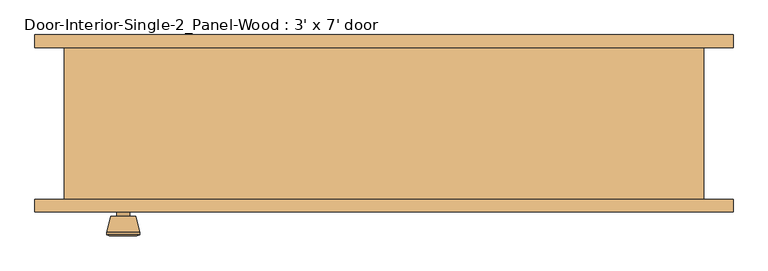
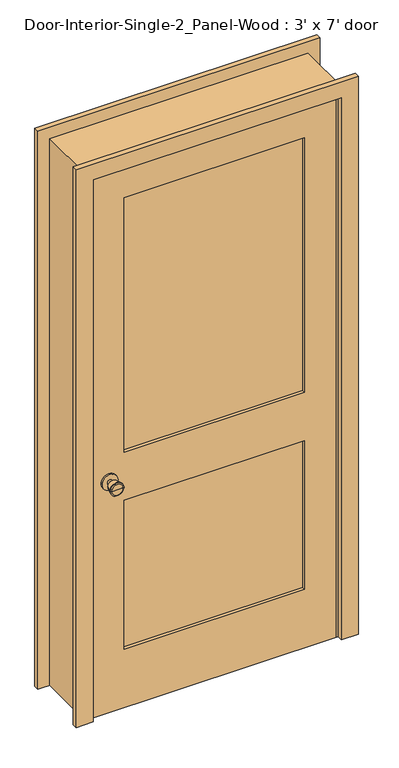
"""IFC4 building model written with IfcOpenShell, lengths in millimetres: door geometry, Door-Interior-Single-2_Panel-Wood : 3' x 7' door."""

from ifc_helpers import new_model, si_unit, point, frame, frame_2d, origin, place, context, project, spatial, polyline, circle_curve, trimmed, segment, composite_curve, outline, extrude, faceted_brep, source, transform, mapped, element, save
from ifc_brep_helpers import plane_surface, cylinder_surface, revolved_surface, advanced_brep


def door_interior_single_2_panel_wood_3_x_7_door_700963f9(model_context):
    return source(origin(), model_context, "Body", "SolidModel", [
        advanced_brep(
        [(-393.7, -70.9, 914.4), (-403.7, -70.9, 914.4), (-383.7, -70.9, 914.4), (-373.2241324, -21.9, 914.4), (-414.1758676, -21.9, 914.4), (-393.7, -21.9, 914.4), (-368.7, -23.7278681, 914.4), (-418.7, -23.7278681, 914.4), (-368.7, -27.1915463, 914.4), (-418.7, -27.1915463, 914.4), (-375.063764, -51.9, 914.4), (-412.336236, -51.9, 914.4), (-383.7, -51.9, 914.4), (-403.7, -51.9, 914.4)],
        [
            (0, 1),
            (1, 2, circle_curve(frame((-393.7, -70.9, 914.4), z_axis=(0.0, -1.0, 0.0), x_axis=(-1.0, 0.0, 0.0)), 10.0)),
            (2, 0),
            (2, 1, circle_curve(frame((-393.7, -70.9, 914.4), z_axis=(0.0, -1.0, 0.0), x_axis=(-1.0, 0.0, 0.0)), 10.0)),
            (3, 4, circle_curve(frame((-393.7, -21.9, 914.4), z_axis=(0.0, 1.0, 0.0), x_axis=(-1.0, 0.0, 0.0)), 20.4758676)),
            (4, 5),
            (5, 3),
            (4, 3, circle_curve(frame((-393.7, -21.9, 914.4), z_axis=(0.0, 1.0, 0.0), x_axis=(-1.0, 0.0, 0.0)), 20.4758676)),
            (6, 7, circle_curve(frame((-393.7, -23.7278681, 914.4), z_axis=(0.0, 1.0, 0.0), x_axis=(-1.0, 0.0, 0.0)), 25.0)),
            (7, 4),
            (3, 6),
            (7, 6, circle_curve(frame((-393.7, -23.7278681, 914.4), z_axis=(0.0, 1.0, 0.0), x_axis=(-1.0, 0.0, 0.0)), 25.0)),
            (8, 9, circle_curve(frame((-393.7, -27.1915463, 914.4), z_axis=(0.0, 1.0, 0.0), x_axis=(-1.0, 0.0, 0.0)), 25.0)),
            (9, 7),
            (6, 8),
            (9, 8, circle_curve(frame((-393.7, -27.1915463, 914.4), z_axis=(0.0, 1.0, 0.0), x_axis=(-1.0, 0.0, 0.0)), 25.0)),
            (10, 11, circle_curve(frame((-393.7, -51.9, 914.4), z_axis=(0.0, 1.0, 0.0), x_axis=(-1.0, 0.0, 0.0)), 18.636236)),
            (11, 9),
            (8, 10),
            (11, 10, circle_curve(frame((-393.7, -51.9, 914.4), z_axis=(0.0, 1.0, 0.0), x_axis=(-1.0, 0.0, 0.0)), 18.636236)),
            (12, 13, circle_curve(frame((-393.7, -51.9, 914.4), z_axis=(0.0, 1.0, 0.0), x_axis=(-1.0, 0.0, 0.0)), 10.0)),
            (13, 11),
            (10, 12),
            (13, 12, circle_curve(frame((-393.7, -51.9, 914.4), z_axis=(0.0, 1.0, 0.0), x_axis=(-1.0, 0.0, 0.0)), 10.0)),
            (1, 13),
            (12, 2),
        ],
        [
            plane_surface(frame((-393.7, -70.9, 914.4), z_axis=(0.0, -1.0, 0.0), x_axis=(-1.0, 0.0, 0.0))),
            plane_surface(frame((-393.7, -21.9, 914.4), z_axis=(0.0, 1.0, 0.0), x_axis=(-1.0, 0.0, 0.0))),
            revolved_surface(polyline([(-414.1758676, -21.9, 914.4), (-418.7, -23.7278681, 914.4)]), (-393.7, -70.9, 914.4), (0.0, -1.0, 0.0)),
            cylinder_surface(frame((-393.7, -70.9, 914.4), z_axis=(0.0, -1.0, 0.0), x_axis=(-1.0, 0.0, 0.0)), 25.0),
            revolved_surface(polyline([(-418.7, -27.1915463, 914.4), (-412.336236, -51.9, 914.4)]), (-393.7, -70.9, 914.4), (0.0, -1.0, 0.0)),
            plane_surface(frame((-393.7, -51.9, 914.4), z_axis=(0.0, -1.0, 0.0), x_axis=(-1.0, 0.0, 0.0))),
            cylinder_surface(frame((-393.7, -70.9, 914.4), z_axis=(0.0, -1.0, 0.0), x_axis=(-1.0, 0.0, 0.0)), 10.0),
        ],
        [
            (0, [[1, 2, 3]]),
            (0, [[-3, 4, -1]]),
            (1, [[5, 6, 7]]),
            (1, [[8, -7, -6]]),
            (2, [[9, 10, -5, 11]]),
            (2, [[12, -11, -8, -10]]),
            (3, [[13, 14, -9, 15]]),
            (3, [[16, -15, -12, -14]]),
            (4, [[17, 18, -13, 19]]),
            (4, [[20, -19, -16, -18]]),
            (5, [[21, 22, -17, 23]]),
            (5, [[24, -23, -20, -22]]),
            (6, [[-2, 25, -21, 26]]),
            (6, [[-4, -26, -24, -25]]),
        ],
    ),
        extrude(outline(composite_curve([segment(trimmed(circle_curve(frame_2d((914.4, -393.7)), 30.0), [point((914.4, -423.7))], [point((914.4, -363.7))], False, "CARTESIAN"), True, "CONTINUOUS"), segment(trimmed(circle_curve(frame_2d((914.4, -393.7)), 30.0), [point((914.4, -363.7))], [point((914.4, -423.7))], False, "CARTESIAN"), True, "CONTINUOUS")], self_intersect=False)), frame((0.0, -76.9, 0.0), z_axis=(0.0, 1.0, 0.0), x_axis=(0.0, 0.0, 1.0)), (0.0, 0.0, 1.0), 6.0),
        advanced_brep(
        [(-393.7, -117.825, 914.4), (-383.7, -117.825, 914.4), (-403.7, -117.825, 914.4), (-373.2241324, -166.825, 914.4), (-393.7, -166.825, 914.4), (-414.1758676, -166.825, 914.4), (-368.7, -164.9971319, 914.4), (-418.7, -164.9971319, 914.4), (-368.7, -161.5334537, 914.4), (-418.7, -161.5334537, 914.4), (-375.063764, -136.825, 914.4), (-412.336236, -136.825, 914.4), (-383.7, -136.825, 914.4), (-403.7, -136.825, 914.4)],
        [
            (0, 1),
            (1, 2, circle_curve(frame((-393.7, -117.825, 914.4), z_axis=(0.0, 1.0, 0.0), x_axis=(-1.0, 0.0, 0.0)), 10.0)),
            (2, 0),
            (2, 1, circle_curve(frame((-393.7, -117.825, 914.4), z_axis=(0.0, 1.0, 0.0), x_axis=(-1.0, 0.0, 0.0)), 10.0)),
            (3, 4),
            (4, 5),
            (5, 3, circle_curve(frame((-393.7, -166.825, 914.4), z_axis=(0.0, -1.0, 0.0), x_axis=(-1.0, 0.0, 0.0)), 20.4758676)),
            (3, 5, circle_curve(frame((-393.7, -166.825, 914.4), z_axis=(0.0, -1.0, 0.0), x_axis=(-1.0, 0.0, 0.0)), 20.4758676)),
            (6, 3),
            (5, 7),
            (7, 6, circle_curve(frame((-393.7, -164.9971319, 914.4), z_axis=(0.0, -1.0, 0.0), x_axis=(-1.0, 0.0, 0.0)), 25.0)),
            (6, 7, circle_curve(frame((-393.7, -164.9971319, 914.4), z_axis=(0.0, -1.0, 0.0), x_axis=(-1.0, 0.0, 0.0)), 25.0)),
            (8, 6),
            (7, 9),
            (9, 8, circle_curve(frame((-393.7, -161.5334537, 914.4), z_axis=(0.0, -1.0, 0.0), x_axis=(-1.0, 0.0, 0.0)), 25.0)),
            (8, 9, circle_curve(frame((-393.7, -161.5334537, 914.4), z_axis=(0.0, -1.0, 0.0), x_axis=(-1.0, 0.0, 0.0)), 25.0)),
            (10, 8),
            (9, 11),
            (11, 10, circle_curve(frame((-393.7, -136.825, 914.4), z_axis=(0.0, -1.0, 0.0), x_axis=(-1.0, 0.0, 0.0)), 18.636236)),
            (10, 11, circle_curve(frame((-393.7, -136.825, 914.4), z_axis=(0.0, -1.0, 0.0), x_axis=(-1.0, 0.0, 0.0)), 18.636236)),
            (12, 10),
            (11, 13),
            (13, 12, circle_curve(frame((-393.7, -136.825, 914.4), z_axis=(0.0, -1.0, 0.0), x_axis=(-1.0, 0.0, 0.0)), 10.0)),
            (12, 13, circle_curve(frame((-393.7, -136.825, 914.4), z_axis=(0.0, -1.0, 0.0), x_axis=(-1.0, 0.0, 0.0)), 10.0)),
            (1, 12),
            (13, 2),
        ],
        [
            plane_surface(frame((-393.7, -117.825, 914.4), z_axis=(0.0, 1.0, 0.0), x_axis=(-1.0, 0.0, 0.0))),
            plane_surface(frame((-393.7, -166.825, 914.4), z_axis=(0.0, -1.0, 0.0), x_axis=(-1.0, 0.0, 0.0))),
            revolved_surface(polyline([(-414.1758676, -166.825, 914.4), (-418.7, -164.9971319, 914.4)]), (-393.7, -117.825, 914.4), (0.0, 1.0, 0.0)),
            cylinder_surface(frame((-393.7, -117.825, 914.4), z_axis=(0.0, 1.0, 0.0), x_axis=(-1.0, 0.0, 0.0)), 25.0),
            revolved_surface(polyline([(-418.7, -161.5334537, 914.4), (-412.336236, -136.825, 914.4)]), (-393.7, -117.825, 914.4), (0.0, 1.0, 0.0)),
            plane_surface(frame((-393.7, -136.825, 914.4), z_axis=(0.0, 1.0, 0.0), x_axis=(-1.0, 0.0, 0.0))),
            cylinder_surface(frame((-393.7, -117.825, 914.4), z_axis=(0.0, 1.0, 0.0), x_axis=(-1.0, 0.0, 0.0)), 10.0),
        ],
        [
            (0, [[1, 2, 3]]),
            (0, [[-3, 4, -1]]),
            (1, [[5, 6, 7]]),
            (1, [[-6, -5, 8]]),
            (2, [[9, -7, 10, 11]]),
            (2, [[-10, -8, -9, 12]]),
            (3, [[13, -11, 14, 15]]),
            (3, [[-14, -12, -13, 16]]),
            (4, [[17, -15, 18, 19]]),
            (4, [[-18, -16, -17, 20]]),
            (5, [[21, -19, 22, 23]]),
            (5, [[-22, -20, -21, 24]]),
            (6, [[25, -23, 26, -2]]),
            (6, [[-26, -24, -25, -4]]),
        ],
    ),
        extrude(outline(composite_curve([segment(trimmed(circle_curve(frame_2d((914.4, -393.7)), 30.0), [point((914.4, -423.7))], [point((914.4, -363.7))], False, "CARTESIAN"), True, "CONTINUOUS"), segment(trimmed(circle_curve(frame_2d((914.4, -393.7)), 30.0), [point((914.4, -363.7))], [point((914.4, -423.7))], False, "CARTESIAN"), True, "CONTINUOUS")], self_intersect=False)), frame((0.0, -117.825, 0.0), z_axis=(0.0, 1.0, 0.0), x_axis=(0.0, 0.0, 1.0)), (0.0, 0.0, 1.0), 6.0),
        faceted_brep([(482.6, -111.825, 0.0), (457.2, -111.825, 0.0), (457.2, -76.9, 0.0), (444.5, -76.9, 0.0), (444.5, -41.975, 0.0), (457.2, -41.975, 0.0), (457.2, 118.175, 0.0), (482.6, 118.175, 0.0), (482.6, 118.175, 2159.0), (482.6, -111.825, 2159.0), (457.2, 118.175, 2133.6), (-457.2, 118.175, 2133.6), (-457.2, 118.175, 0.0), (-482.6, 118.175, 0.0), (-482.6, 118.175, 2159.0), (457.2, -41.975, 2133.6), (444.5, -41.975, 2120.9), (-444.5, -41.975, 2120.9), (-444.5, -41.975, 0.0), (-457.2, -41.975, 0.0), (-457.2, -41.975, 2133.6), (444.5, -76.9, 2120.9), (457.2, -76.9, 2133.6), (-457.2, -76.9, 2133.6), (-457.2, -76.9, 0.0), (-444.5, -76.9, 0.0), (-444.5, -76.9, 2120.9), (457.2, -111.825, 2133.6), (-482.6, -111.825, 2159.0), (-482.6, -111.825, 0.0), (-457.2, -111.825, 0.0), (-457.2, -111.825, 2133.6)], [[[0, 1, 2, 3, 4, 5, 6, 7]], [[7, 8, 9, 0]], [[6, 10, 11, 12, 13, 14, 8, 7]], [[5, 15, 10, 6]], [[4, 16, 17, 18, 19, 20, 15, 5]], [[3, 21, 16, 4]], [[2, 22, 23, 24, 25, 26, 21, 3]], [[1, 27, 22, 2]], [[0, 9, 28, 29, 30, 31, 27, 1]], [[8, 14, 28, 9]], [[15, 20, 11, 10]], [[21, 26, 17, 16]], [[27, 31, 23, 22]], [[29, 13, 12, 19, 18, 25, 24, 30]], [[14, 13, 29, 28]], [[20, 19, 12, 11]], [[26, 25, 18, 17]], [[31, 30, 24, 23]]]),
        extrude(outline(polyline([(2133.6, -457.2), (0.0, -457.2), (0.0, 457.2), (2133.6, 457.2), (2133.6, -457.2)]), holes=[polyline([(2014.5375, -336.55), (2014.5375, 336.55), (1009.65, 336.55), (1009.65, -336.55), (2014.5375, -336.55)]), polyline([(819.15, -336.55), (819.15, 336.55), (231.775, 336.55), (231.775, -336.55), (819.15, -336.55)])]), frame((0.0, -111.825, 0.0), z_axis=(0.0, 1.0, 0.0), x_axis=(0.0, 0.0, 1.0)), (0.0, 0.0, 1.0), 34.925),
        extrude(outline(polyline([(336.55, -88.5416667), (336.55, -100.1833333), (-336.55, -100.1833333), (-336.55, -88.5416667), (336.55, -88.5416667)])), frame((0.0, 0.0, 1009.65), z_axis=(0.0, 0.0, 1.0), x_axis=(1.0, 0.0, 0.0)), (0.0, 0.0, 1.0), 1004.8875),
        extrude(outline(polyline([(336.55, -88.5416667), (336.55, -100.1833333), (-336.55, -100.1833333), (-336.55, -88.5416667), (336.55, -88.5416667)])), frame((0.0, 0.0, 231.775), z_axis=(0.0, 0.0, 1.0), x_axis=(1.0, 0.0, 0.0)), (0.0, 0.0, 1.0), 587.375),
        extrude(outline(polyline([(0.0, 527.05), (2203.45, 527.05), (2203.45, -527.05), (0.0, -527.05), (0.0, -463.55), (2139.95, -463.55), (2139.95, 463.55), (0.0, 463.55), (0.0, 527.05)])), frame((0.0, -130.875, 0.0), z_axis=(0.0, 1.0, 0.0), x_axis=(0.0, 0.0, 1.0)), (0.0, 0.0, 1.0), 19.05),
        extrude(outline(polyline([(0.0, 527.05), (2203.45, 527.05), (2203.45, -527.05), (0.0, -527.05), (0.0, -463.55), (2139.95, -463.55), (2139.95, 463.55), (0.0, 463.55), (0.0, 527.05)])), frame((0.0, 118.175, 0.0), z_axis=(0.0, 1.0, 0.0), x_axis=(0.0, 0.0, 1.0)), (0.0, 0.0, 1.0), 19.05),
    ])


if __name__ == "__main__":
    model = new_model("IFC4")
    model_context = context("Model", 3, world=origin())
    ifc_project = project(units=[si_unit("LENGTHUNIT", "METRE", prefix="MILLI")], contexts=[model_context])
    site = spatial("IfcSite", under=ifc_project)
    building = spatial("IfcBuilding", under=site)
    placement = place(None, origin())
    door_interior_single_2_panel_wood_3_x_7_door_shape = door_interior_single_2_panel_wood_3_x_7_door_700963f9(model_context)
    element("IfcDoor", 1, ObjectType="Door-Interior-Single-2_Panel-Wood : 3' x 7' door", at=placement, inside=building, context=model_context, shape_type="MappedRepresentation", body=[
        mapped(door_interior_single_2_panel_wood_3_x_7_door_shape, transform((0.0, 0.0, 0.0), x_axis=(1.0, 0.0, 0.0), y_axis=(0.0, 1.0, 0.0), z_axis=(0.0, 0.0, 1.0))),
    ])
    save(model, "model.ifc")

# Revit data of these elements
# Type "Door-Interior-Single-2_Panel-Wood : 3' x 7' door"
#   Type Mark = "9"
#   Assembly Code = "C1020300"
#   Analytic Construction = "Wooden"
#   Top Rail = 0' - 4 11/16"
#   Thickness = 0' - 1 3/8"
#   Thermal Resistance (R) = 2.5876 (h·ft²·°F)/BTU
#   Swing Angle [instance default] = 90.00°
#   Stiles = 0' - 4 3/4"
#   Rough Width = 3' - 2"
#   Rough Height = 7' - 1"
#   Lock Rail = 0' - 7 1/2"
#   Height = 7' - 0"
#   Width = 3' - 0"
#   Heat Transfer Coefficient (U) = 0.3865 BTU/(h·ft²·°F)
#   Bottom Rail = 0' - 9 1/8"
#   Trim Material = Cherry
#   Panel Material = Cherry
#   Frame Material = Cherry
#   Door Handle Material = Aluminum
#   Visual Light Transmittance = 0
#   Solar Heat Gain Coefficient = 0
#   Wall Closure = (empty or 0)
#   Function = (empty or 0)
# Element 1 (IfcDoor, "Door-Interior-Single-2_Panel-Wood : 3' x 7' door")
#   Materials on its faces: "Cherry", "Aluminum"
# Materials
#   "Cherry": class "Wood", colour RGB 226 177 128, transparency 0, Description = "Prunus Serotina", Cost = 0
#   "Aluminum": class "Metal", colour RGB 247 247 247, transparency 0, Description = "Aluminum 6061", Cost = 0
